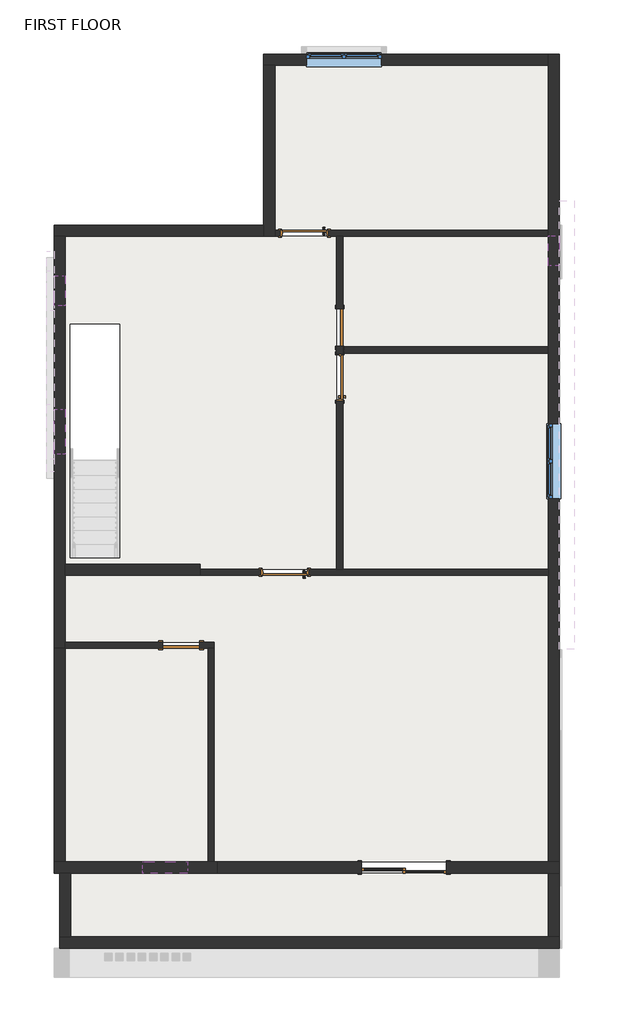
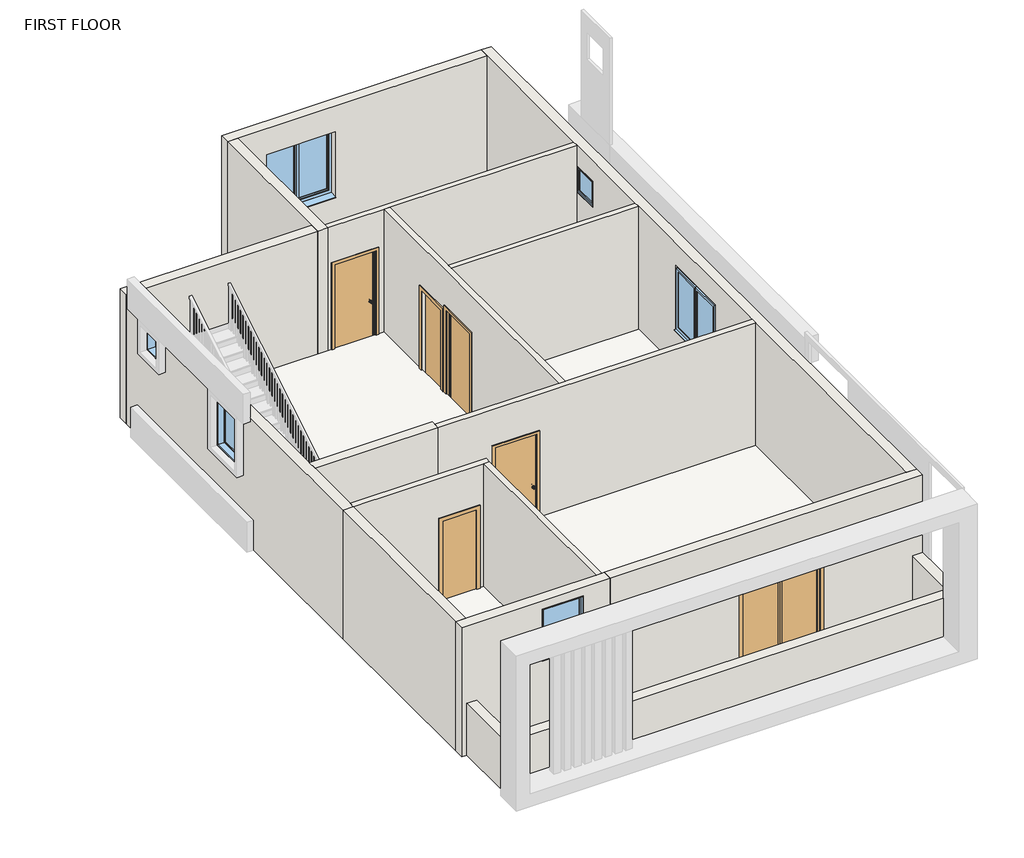
# One storey, part 1 of 2: 18 walls, 6 doors, 6 windows, 1 slab.
"""IFC4 building model written with IfcOpenShell, lengths in millimetres."""

from ifc_helpers import new_model, si_unit, frame, origin, place, context, project, spatial, polyline, outline, extrude, faceted_brep, transform, mapped, element, save
from components import door_45189e27, door_92402058, door_fdc9072e, door_1fe7f57d, window_80340324, fixed_window_3_x_3_dcb239d8, w2_windows_5_x_5_8ac21896

model = new_model("IFC4")

# Units and contexts
model_context = context("Model", 3, world=origin())
ifc_project = project(units=[si_unit("LENGTHUNIT", "METRE", prefix="MILLI")], contexts=[model_context])

# Site, building, storey
site = spatial("IfcSite", under=ifc_project)
building = spatial("IfcBuilding", under=site)
storey = spatial("IfcBuildingStorey", under=building, Name="FIRST FLOOR", Elevation=3352.8)

# Doors
placement = place(None, origin())
door_shape = door_45189e27(model_context)
element("IfcDoor", 1, ObjectType="Door-Double-Sliding : 68\" x 84\"", at=placement, inside=storey, context=model_context, shape_type="MappedRepresentation", body=[
    mapped(door_shape, transform((1027.2719693, -4152.8358748, 3352.8), x_axis=(-1.0, 0.0, 0.0), y_axis=(0.0, -1.0, 0.0), z_axis=(0.0, 0.0, 1.0))),
])
door_2_shape = door_92402058(model_context)
element("IfcDoor", 2, ObjectType="Door-Interior-Single-Flush_Panel-Wood : 36\" x 84\"", at=placement, inside=storey, context=model_context, shape_type="MappedRepresentation", body=[
    mapped(door_2_shape, transform((-1398.4280307, 1724.0891252, 3352.8), x_axis=(-1.0, 0.0, 0.0), y_axis=(0.0, -1.0, 0.0), z_axis=(0.0, 0.0, 1.0))),
])
door_3_shape = door_fdc9072e(model_context)
element("IfcDoor", 3, ObjectType="Door-Interior-Single-Flush_Panel-Wood : 36\" x 84\"", at=placement, inside=storey, context=model_context, shape_type="MappedRepresentation", body=[
    mapped(door_3_shape, transform((-998.3780307, 8626.5391252, 3352.8), x_axis=(-1.0, 0.0, 0.0), y_axis=(0.0, -1.0, 0.0), z_axis=(0.0, 0.0, 1.0))),
])
element("IfcDoor", 4, ObjectType="Door-Interior-Single-Flush_Panel-Wood : 36\" x 84\"", at=placement, inside=storey, context=model_context, shape_type="MappedRepresentation", body=[
    mapped(door_3_shape, transform((-277.6530307, 5689.6641252, 3352.8), x_axis=(0.0, 1.0, 0.0), y_axis=(-1.0, 0.0, 0.0), z_axis=(0.0, 0.0, 1.0))),
])
door_4_shape = door_1fe7f57d(model_context)
element("IfcDoor", 5, ObjectType="Single-Flush : 30\" x 80\"", at=placement, inside=storey, context=model_context, shape_type="MappedRepresentation", body=[
    mapped(door_4_shape, transform((-3509.8822467, 241.3641252, 3352.8), x_axis=(-1.0, 0.0, 0.0), y_axis=(0.0, -1.0, 0.0), z_axis=(0.0, 0.0, 1.0))),
])
element("IfcDoor", 6, ObjectType="Single-Flush : 30\" x 80\"", at=placement, inside=storey, context=model_context, shape_type="MappedRepresentation", body=[
    mapped(door_4_shape, transform((-280.8280307, 6705.6641252, 3352.8), x_axis=(0.0, -1.0, 0.0), y_axis=(1.0, 0.0, 0.0), z_axis=(0.0, 0.0, 1.0))),
])

# Slab
element("IfcSlab", 7, ObjectType="MARBLE 6\"", at=placement, inside=storey, context=model_context, shape_type="SweptSolid", body=[
    extrude(outline(polyline([(-2963.7822467, -4165.5358748), (-5868.7932997, -4165.5358748), (-5868.7932997, 177.8641252), (-2963.7822467, 177.8641252), (-2963.7822467, -4165.5358748)])), frame((0.0, 0.0, 3352.8), z_axis=(0.0, 0.0, 1.0), x_axis=(1.0, 0.0, 0.0)), (0.0, 0.0, 1.0), 152.4),
    extrude(outline(polyline([(-217.3280307, 6184.9641252), (3960.9719693, 6184.9641252), (3960.9719693, 1790.7641252), (-217.3280307, 1790.7641252), (-217.3280307, 6184.9641252)])), frame((0.0, 0.0, 3352.8), z_axis=(0.0, 0.0, 1.0), x_axis=(1.0, 0.0, 0.0)), (0.0, 0.0, 1.0), 152.4),
    extrude(outline(polyline([(-1601.6280307, 12039.6641252), (3960.9719693, 12039.6641252), (3960.9719693, 8686.8641252), (-1601.6280307, 8686.8641252), (-1601.6280307, 12039.6641252)])), frame((0.0, 0.0, 3352.8), z_axis=(0.0, 0.0, 1.0), x_axis=(1.0, 0.0, 0.0)), (0.0, 0.0, 1.0), 152.4),
    extrude(outline(polyline([(-217.3280307, 8559.8641252), (3960.9719693, 8559.8641252), (3960.9719693, 6311.9641252), (-217.3280307, 6311.9641252), (-217.3280307, 8559.8641252)])), frame((0.0, 0.0, 3352.8), z_axis=(0.0, 0.0, 1.0), x_axis=(1.0, 0.0, 0.0)), (0.0, 0.0, 1.0), 152.4),
    extrude(outline(polyline([(3960.9719693, -4394.1358748), (3960.9719693, -5689.5358748), (-5868.7932997, -5689.5358748), (-5868.7932997, -4394.1358748), (3960.9719693, -4394.1358748)])), frame((0.0, 0.0, 3352.8), z_axis=(0.0, 0.0, 1.0), x_axis=(1.0, 0.0, 0.0)), (0.0, 0.0, 1.0), 152.4),
    extrude(outline(polyline([(-344.3280307, 8559.8641252), (-344.3280307, 1790.7641252), (-5868.8280307, 1790.7641252), (-5868.8280307, 8559.8641252), (-344.3280307, 8559.8641252)]), holes=[polyline([(-4756.3875748, 6770.5325341), (-5772.3875748, 6770.5325341), (-5772.3875748, 2020.7325341), (-4756.3875748, 2020.7325341), (-4756.3875748, 6770.5325341)])]), frame((0.0, 0.0, 3352.8), z_axis=(0.0, 0.0, 1.0), x_axis=(1.0, 0.0, 0.0)), (0.0, 0.0, 1.0), 152.4),
    extrude(outline(polyline([(3960.9719693, 1663.7641252), (3960.9719693, -4165.5358748), (-2836.7822467, -4165.5358748), (-2836.7822467, 304.8641252), (-5868.8280307, 304.8641252), (-5868.8280307, 1663.7641252), (3960.9719693, 1663.7641252)])), frame((0.0, 0.0, 3352.8), z_axis=(0.0, 0.0, 1.0), x_axis=(1.0, 0.0, 0.0)), (0.0, 0.0, 1.0), 152.4),
])

# Walls
element("IfcWall", 8, ObjectType="INNER WALL5\"", at=placement, inside=storey, context=model_context, shape_type="Brep", body=[
    faceted_brep([(3960.9719693, 8559.8641252, 6400.8), (-217.3280307, 8559.8641252, 6400.8), (-344.3280307, 8559.8641252, 6400.8), (-1601.6280307, 8559.8641252, 6400.8), (-1601.6280307, 8559.8641252, 3352.8), (-1480.9780307, 8559.8641252, 3352.8), (-1480.9780307, 8559.8641252, 5511.8), (-515.7780307, 8559.8641252, 5511.8), (-515.7780307, 8559.8641252, 3352.8), (-344.3280307, 8559.8641252, 3352.8), (-217.3280307, 8559.8641252, 3352.8), (3960.9719693, 8559.8641252, 3352.8), (-1601.6280307, 8686.8641252, 6400.8), (3960.9719693, 8686.8641252, 6400.8), (3960.9719693, 8686.8641252, 3352.8), (-515.7780307, 8686.8641252, 3352.8), (-515.7780307, 8686.8641252, 5511.8), (-1480.9780307, 8686.8641252, 5511.8), (-1480.9780307, 8686.8641252, 3352.8), (-1601.6280307, 8686.8641252, 3352.8)], [[[0, 1, 2, 3, 4, 5, 6, 7, 8, 9, 10, 11]], [[12, 13, 14, 15, 16, 17, 18, 19]], [[14, 11, 10, 9, 8, 15]], [[4, 19, 18, 5]], [[3, 2, 1, 0, 13, 12]], [[0, 11, 14, 13]], [[4, 3, 12, 19]], [[17, 6, 5, 18]], [[6, 17, 16, 7]], [[7, 16, 15, 8]]]),
])
element("IfcWall", 9, ObjectType="INNER WALL5\"", at=placement, inside=storey, context=model_context, shape_type="Brep", body=[
    faceted_brep([(-5868.7932997, 177.8641252, 3352.8), (-3890.8822467, 177.8641252, 3352.8), (-3890.8822467, 177.8641252, 5384.8), (-3128.8822467, 177.8641252, 5384.8), (-3128.8822467, 177.8641252, 3352.8), (-2963.7822467, 177.8641252, 3352.8), (-2836.7822467, 177.8641252, 3352.8), (-2836.7822467, 177.8641252, 6400.8), (-2963.7822467, 177.8641252, 6400.8), (-5868.7932997, 177.8641252, 6400.8), (-3890.8822467, 304.8641252, 5384.8), (-3890.8822467, 304.8641252, 3352.8), (-5868.7932997, 304.8641252, 3352.8), (-5868.7932997, 304.8641252, 6400.8), (-2836.7822467, 304.8641252, 6400.8), (-2836.7822467, 304.8641252, 3352.8), (-3128.8822467, 304.8641252, 3352.8), (-3128.8822467, 304.8641252, 5384.8)], [[[0, 1, 2, 3, 4, 5, 6, 7, 8, 9]], [[10, 11, 12, 13, 14, 15, 16, 17]], [[16, 15, 6, 5, 4]], [[12, 11, 1, 0]], [[9, 8, 7, 14, 13]], [[7, 6, 15, 14]], [[2, 1, 11, 10]], [[3, 2, 10, 17]], [[4, 3, 17, 16]], [[0, 9, 13, 12]]]),
])
element("IfcWall", 10, ObjectType="INNER WALL5\"", at=placement, inside=storey, context=model_context, shape_type="SweptSolid", body=[
    extrude(outline(polyline([(-2963.7822467, -4165.5358748), (-2963.7822467, 177.8641252), (-2836.7822467, 177.8641252), (-2836.7822467, -4165.5358748), (-2963.7822467, -4165.5358748)])), frame((0.0, 0.0, 3352.8), z_axis=(0.0, 0.0, 1.0), x_axis=(1.0, 0.0, 0.0)), (0.0, 0.0, 1.0), 3048.0),
])
element("IfcWall", 11, ObjectType="INNER WALL5\"", at=placement, inside=storey, context=model_context, shape_type="Brep", body=[
    faceted_brep([(3960.9719693, 1663.7641252, 6400.8), (-3125.6280307, 1663.7641252, 6400.8), (-3125.6280307, 1663.7641252, 3352.8), (-1881.0280307, 1663.7641252, 3352.8), (-1881.0280307, 1663.7641252, 5511.8), (-915.8280307, 1663.7641252, 5511.8), (-915.8280307, 1663.7641252, 3352.8), (3960.9719693, 1663.7641252, 3352.8), (-3125.6280307, 1790.7641252, 6400.8), (-344.3280307, 1790.7641252, 6400.8), (-217.3280307, 1790.7641252, 6400.8), (3960.9719693, 1790.7641252, 6400.8), (3960.9719693, 1790.7641252, 3352.8), (-217.3280307, 1790.7641252, 3352.8), (-344.3280307, 1790.7641252, 3352.8), (-915.8280307, 1790.7641252, 3352.8), (-915.8280307, 1790.7641252, 5511.8), (-1881.0280307, 1790.7641252, 5511.8), (-1881.0280307, 1790.7641252, 3352.8), (-3125.6280307, 1790.7641252, 3352.8)], [[[0, 1, 2, 3, 4, 5, 6, 7]], [[8, 9, 10, 11, 12, 13, 14, 15, 16, 17, 18, 19]], [[2, 19, 18, 3]], [[12, 7, 6, 15, 14, 13]], [[1, 0, 11, 10, 9, 8]], [[2, 1, 8, 19]], [[0, 7, 12, 11]], [[17, 4, 3, 18]], [[4, 17, 16, 5]], [[5, 16, 15, 6]]]),
])
element("IfcWall", 12, ObjectType="INNER WALL5\"", at=placement, inside=storey, context=model_context, shape_type="Brep", body=[
    faceted_brep([(-344.3280307, 1790.7641252, 6400.8), (-344.3280307, 8559.8641252, 6400.8), (-344.3280307, 8559.8641252, 3352.8), (-344.3280307, 7086.6641252, 3352.8), (-344.3280307, 7086.6641252, 5384.8), (-344.3280307, 6324.6641252, 5384.8), (-344.3280307, 6324.6641252, 3352.8), (-344.3280307, 6172.2641252, 3352.8), (-344.3280307, 6172.2641252, 5511.8), (-344.3280307, 5207.0641252, 5511.8), (-344.3280307, 5207.0641252, 3352.8), (-344.3280307, 1790.7641252, 3352.8), (-217.3280307, 8559.8641252, 6400.8), (-217.3280307, 6311.9641252, 6400.8), (-217.3280307, 6184.9641252, 6400.8), (-217.3280307, 1790.7641252, 6400.8), (-217.3280307, 1790.7641252, 3352.8), (-217.3280307, 5207.0641252, 3352.8), (-217.3280307, 5207.0641252, 5511.8), (-217.3280307, 6172.2641252, 5511.8), (-217.3280307, 6172.2641252, 3352.8), (-217.3280307, 6184.9641252, 3352.8), (-217.3280307, 6311.9641252, 3352.8), (-217.3280307, 6324.6641252, 3352.8), (-217.3280307, 6324.6641252, 5384.8), (-217.3280307, 7086.6641252, 5384.8), (-217.3280307, 7086.6641252, 3352.8), (-217.3280307, 8559.8641252, 3352.8)], [[[0, 1, 2, 3, 4, 5, 6, 7, 8, 9, 10, 11]], [[12, 13, 14, 15, 16, 17, 18, 19, 20, 21, 22, 23, 24, 25, 26, 27]], [[2, 27, 26, 3]], [[16, 11, 10, 17]], [[6, 23, 22, 21, 20, 7]], [[1, 0, 15, 14, 13, 12]], [[2, 1, 12, 27]], [[0, 11, 16, 15]], [[24, 23, 6, 5]], [[25, 24, 5, 4]], [[26, 25, 4, 3]], [[19, 8, 7, 20]], [[8, 19, 18, 9]], [[9, 18, 17, 10]]]),
])
element("IfcWall", 13, ObjectType="INNER WALL5\"", at=placement, inside=storey, context=model_context, shape_type="SweptSolid", body=[
    extrude(outline(polyline([(3960.9719693, 6184.9641252), (-217.3280307, 6184.9641252), (-217.3280307, 6311.9641252), (3960.9719693, 6311.9641252), (3960.9719693, 6184.9641252)])), frame((0.0, 0.0, 3352.8), z_axis=(0.0, 0.0, 1.0), x_axis=(1.0, 0.0, 0.0)), (0.0, 0.0, 1.0), 3048.0),
])
element("IfcWall", 14, ObjectType="OUTER WALL 9\"", at=placement, inside=storey, context=model_context, shape_type="Brep", body=[
    faceted_brep([(4189.5719693, -4165.5358748, 6400.8), (4189.5719693, -4165.5358748, 3352.8), (4189.5719693, 12268.2641252, 3352.8), (4189.5719693, 12268.2641252, 6400.8), (4189.5719693, 4749.8641252, 4352.8), (4189.5719693, 3225.8641252, 4352.8), (4189.5719693, 3225.8641252, 5876.8), (4189.5719693, 4749.8641252, 5876.8), (4189.5719693, 8572.5641252, 5908.2819261), (4189.5719693, 8572.5641252, 5298.6819261), (4189.5719693, 7962.9641252, 5298.6819261), (4189.5719693, 7962.9641252, 5908.2819261), (3960.9719693, -4165.5358748, 3352.8), (3960.9719693, -4165.5358748, 6400.8), (3960.9719693, 1663.7641252, 6400.8), (3960.9719693, 1790.7641252, 6400.8), (3960.9719693, 6184.9641252, 6400.8), (3960.9719693, 6311.9641252, 6400.8), (3960.9719693, 8559.8641252, 6400.8), (3960.9719693, 8686.8641252, 6400.8), (3960.9719693, 12039.6641252, 6400.8), (3960.9719693, 12268.2641252, 6400.8), (3960.9719693, 12268.2641252, 3352.8), (3960.9719693, 12039.6641252, 3352.8), (3960.9719693, 8686.8641252, 3352.8), (3960.9719693, 8559.8641252, 3352.8), (3960.9719693, 6311.9641252, 3352.8), (3960.9719693, 6184.9641252, 3352.8), (3960.9719693, 1790.7641252, 3352.8), (3960.9719693, 1663.7641252, 3352.8), (3960.9719693, 4749.8641252, 4352.8), (3960.9719693, 4749.8641252, 5876.8), (3960.9719693, 3225.8641252, 5876.8), (3960.9719693, 3225.8641252, 4352.8), (3960.9719693, 8572.5641252, 5908.2819261), (3960.9719693, 7962.9641252, 5908.2819261), (3960.9719693, 7962.9641252, 5298.6819261), (3960.9719693, 8572.5641252, 5298.6819261)], [[[0, 1, 2, 3], [4, 5, 6, 7], [8, 9, 10, 11]], [[12, 13, 14, 15, 16, 17, 18, 19, 20, 21, 22, 23, 24, 25, 26, 27, 28, 29], [30, 31, 32, 33], [34, 35, 36, 37]], [[2, 1, 12, 29, 28, 27, 26, 25, 24, 23, 22]], [[0, 3, 21, 20, 19, 18, 17, 16, 15, 14, 13]], [[3, 2, 22, 21]], [[0, 13, 12, 1]], [[31, 30, 4, 7]], [[32, 31, 7, 6]], [[33, 32, 6, 5]], [[30, 33, 5, 4]], [[9, 8, 34, 37]], [[10, 9, 37, 36]], [[11, 10, 36, 35]], [[8, 11, 35, 34]]]),
])
element("IfcWall", 15, ObjectType="OUTER WALL 9\"", at=placement, inside=storey, context=model_context, shape_type="Brep", body=[
    faceted_brep([(3960.9719693, 12268.2641252, 3352.8), (-1830.2280307, 12268.2641252, 3352.8), (-1830.2280307, 12268.2641252, 6400.8), (3960.9719693, 12268.2641252, 6400.8), (570.0719693, 12268.2641252, 4267.2), (570.0719693, 12268.2641252, 5791.2), (-953.9280307, 12268.2641252, 5791.2), (-953.9280307, 12268.2641252, 4267.2), (3960.9719693, 12039.6641252, 3352.8), (3960.9719693, 12039.6641252, 6400.8), (-1601.6280307, 12039.6641252, 6400.8), (-1830.2280307, 12039.6641252, 6400.8), (-1830.2280307, 12039.6641252, 3352.8), (-1601.6280307, 12039.6641252, 3352.8), (570.0719693, 12039.6641252, 4267.2), (-953.9280307, 12039.6641252, 4267.2), (-953.9280307, 12039.6641252, 5791.2), (570.0719693, 12039.6641252, 5791.2)], [[[0, 1, 2, 3], [4, 5, 6, 7]], [[8, 9, 10, 11, 12, 13], [14, 15, 16, 17]], [[1, 0, 8, 13, 12]], [[3, 2, 11, 10, 9]], [[0, 3, 9, 8]], [[2, 1, 12, 11]], [[5, 4, 14, 17]], [[6, 5, 17, 16]], [[7, 6, 16, 15]], [[4, 7, 15, 14]]]),
])
element("IfcWall", 16, ObjectType="OUTER WALL 9\"", at=placement, inside=storey, context=model_context, shape_type="Brep", body=[
    faceted_brep([(-1830.2280307, 12039.6641252, 3352.8), (-1830.2280307, 8788.4641252, 3352.8), (-1830.2280307, 8559.8641252, 3352.8), (-1830.2280307, 8559.8641252, 6400.8), (-1830.2280307, 8788.4641252, 6400.8), (-1830.2280307, 12039.6641252, 6400.8), (-1601.6280307, 12039.6641252, 3352.8), (-1601.6280307, 12039.6641252, 6400.8), (-1601.6280307, 8686.8641252, 6400.8), (-1601.6280307, 8559.8641252, 6400.8), (-1601.6280307, 8559.8641252, 3352.8), (-1601.6280307, 8686.8641252, 3352.8)], [[[0, 1, 2, 3, 4, 5]], [[6, 7, 8, 9, 10, 11]], [[2, 1, 0, 6, 11, 10]], [[5, 4, 3, 9, 8, 7]], [[0, 5, 7, 6]], [[3, 2, 10, 9]]]),
])
element("IfcWall", 17, ObjectType="OUTER WALL 9\"", at=placement, inside=storey, context=model_context, shape_type="Brep", body=[
    faceted_brep([(-1830.2280307, 8788.4641252, 3352.8), (-6097.3932997, 8788.4641252, 3352.8), (-6097.3932997, 8788.4641252, 6400.8), (-1830.2280307, 8788.4641252, 6400.8), (-1830.2280307, 8559.8641252, 3352.8), (-1830.2280307, 8559.8641252, 6400.8), (-5868.7932997, 8559.8641252, 6400.8), (-6097.3932997, 8559.8641252, 6400.8), (-6097.3932997, 8559.8641252, 3352.8), (-5868.7932997, 8559.8641252, 3352.8)], [[[0, 1, 2, 3]], [[4, 5, 6, 7, 8, 9]], [[1, 0, 4, 9, 8]], [[3, 2, 7, 6, 5]], [[0, 3, 5, 4]], [[2, 1, 8, 7]]]),
])
element("IfcWall", 18, ObjectType="OUTER WALL 9\"", at=placement, inside=storey, context=model_context, shape_type="Brep", body=[
    faceted_brep([(-6097.3932997, 8559.8641252, 3352.8), (-6097.3932997, 177.8641252, 3352.8), (-6097.3932997, 177.8641252, 6400.8), (-6097.3932997, 8559.8641252, 6400.8), (-6097.3932997, 7150.1641252, 6189.9849297), (-6097.3932997, 7150.1641252, 5580.3849297), (-6097.3932997, 7759.7641252, 5580.3849297), (-6097.3932997, 7759.7641252, 6189.9849297), (-6097.3932997, 4127.5641252, 6204.2433359), (-6097.3932997, 4127.5641252, 4985.0433359), (-6097.3932997, 5041.9641252, 4985.0433359), (-6097.3932997, 5041.9641252, 6204.2433359), (-5868.7932997, 8559.8641252, 3352.8), (-5868.7932997, 8559.8641252, 6400.8), (-5868.7932997, 1892.3641252, 6400.8), (-5868.7932997, 1663.7641252, 6400.8), (-5868.7932997, 304.8641252, 6400.8), (-5868.7932997, 177.8641252, 6400.8), (-5868.7932997, 177.8641252, 3352.8), (-5868.7932997, 304.8641252, 3352.8), (-5868.7932997, 1663.7641252, 3352.8), (-5868.7932997, 1892.3641252, 3352.8), (-5868.7932997, 7150.1641252, 6189.9849297), (-5868.7932997, 7759.7641252, 6189.9849297), (-5868.7932997, 7759.7641252, 5580.3849297), (-5868.7932997, 7150.1641252, 5580.3849297), (-5868.7932997, 4127.5641252, 6204.2433359), (-5868.7932997, 5041.9641252, 6204.2433359), (-5868.7932997, 5041.9641252, 4985.0433359), (-5868.7932997, 4127.5641252, 4985.0433359)], [[[0, 1, 2, 3], [4, 5, 6, 7], [8, 9, 10, 11]], [[12, 13, 14, 15, 16, 17, 18, 19, 20, 21], [22, 23, 24, 25], [26, 27, 28, 29]], [[1, 0, 12, 21, 20, 19, 18]], [[3, 2, 17, 16, 15, 14, 13]], [[0, 3, 13, 12]], [[2, 1, 18, 17]], [[5, 4, 22, 25]], [[6, 5, 25, 24]], [[7, 6, 24, 23]], [[4, 7, 23, 22]], [[9, 8, 26, 29]], [[10, 9, 29, 28]], [[11, 10, 28, 27]], [[8, 11, 27, 26]]]),
])
element("IfcWall", 19, ObjectType="OUTER WALL 9\"", at=placement, inside=storey, context=model_context, shape_type="Brep", body=[
    faceted_brep([(-2782.7280307, -4394.1358748, 3352.8), (163.6719693, -4394.1358748, 3352.8), (163.6719693, -4394.1358748, 5486.4), (1890.8719693, -4394.1358748, 5486.4), (1890.8719693, -4394.1358748, 3352.8), (3960.9719693, -4394.1358748, 3352.8), (4189.5719693, -4394.1358748, 3352.8), (4189.5719693, -4394.1358748, 4572.0), (4189.5719693, -4394.1358748, 6400.8), (-2782.7280307, -4394.1358748, 6400.8), (163.6719693, -4165.5358748, 5486.4), (163.6719693, -4165.5358748, 3352.8), (-2782.7280307, -4165.5358748, 3352.8), (-2782.7280307, -4165.5358748, 6400.8), (3960.9719693, -4165.5358748, 6400.8), (4189.5719693, -4165.5358748, 6400.8), (4189.5719693, -4165.5358748, 3352.8), (3960.9719693, -4165.5358748, 3352.8), (1890.8719693, -4165.5358748, 3352.8), (1890.8719693, -4165.5358748, 5486.4)], [[[0, 1, 2, 3, 4, 5, 6, 7, 8, 9]], [[10, 11, 12, 13, 14, 15, 16, 17, 18, 19]], [[12, 11, 1, 0]], [[18, 17, 16, 6, 5, 4]], [[9, 8, 15, 14, 13]], [[0, 9, 13, 12]], [[6, 16, 15, 8, 7]], [[4, 3, 19, 18]], [[2, 1, 11, 10]], [[3, 2, 10, 19]]]),
])
element("IfcWall", 20, ObjectType="OUTER WALL 9\"", at=placement, inside=storey, context=model_context, shape_type="Brep", body=[
    faceted_brep([(-2782.7280307, -4165.5358748, 3352.8), (-2836.7822467, -4165.5358748, 3352.8), (-2963.7822467, -4165.5358748, 3352.8), (-5868.7932997, -4165.5358748, 3352.8), (-6097.3932997, -4165.5358748, 3352.8), (-6097.3932997, -4165.5358748, 6400.8), (-5868.7932997, -4165.5358748, 6400.8), (-2963.7822467, -4165.5358748, 6400.8), (-2836.7822467, -4165.5358748, 6400.8), (-2782.7280307, -4165.5358748, 6400.8), (-4294.0280307, -4165.5358748, 6197.6), (-4294.0280307, -4165.5358748, 4978.4), (-3379.6280307, -4165.5358748, 4978.4), (-3379.6280307, -4165.5358748, 6197.6), (-2782.7280307, -4394.1358748, 3352.8), (-2782.7280307, -4394.1358748, 6400.8), (-6097.3932997, -4394.1358748, 6400.8), (-6097.3932997, -4394.1358748, 3352.8), (-5983.1280307, -4394.1358748, 3352.8), (-5754.5280307, -4394.1358748, 3352.8), (-4294.0280307, -4394.1358748, 6197.6), (-3379.6280307, -4394.1358748, 6197.6), (-3379.6280307, -4394.1358748, 4978.4), (-4294.0280307, -4394.1358748, 4978.4)], [[[0, 1, 2, 3, 4, 5, 6, 7, 8, 9], [10, 11, 12, 13]], [[14, 15, 16, 17, 18, 19], [20, 21, 22, 23]], [[4, 3, 2, 1, 0, 14, 19, 18, 17]], [[9, 8, 7, 6, 5, 16, 15]], [[0, 9, 15, 14]], [[11, 10, 20, 23]], [[12, 11, 23, 22]], [[13, 12, 22, 21]], [[10, 13, 21, 20]], [[4, 17, 16, 5]]]),
])
element("IfcWall", 21, ObjectType="OUTER WALL 9\"", at=placement, inside=storey, context=model_context, shape_type="Brep", body=[
    faceted_brep([(-5983.1280307, -5918.1358748, 3352.8), (4189.5719693, -5918.1358748, 3352.8), (4189.5719693, -5918.1358748, 4572.0), (-5983.1280307, -5918.1358748, 4572.0), (-5983.1280307, -5689.5358748, 3352.8), (-5983.1280307, -5689.5358748, 4572.0), (-5754.5280307, -5689.5358748, 4572.0), (3960.9719693, -5689.5358748, 4572.0), (4189.5719693, -5689.5358748, 4572.0), (4189.5719693, -5689.5358748, 3352.8), (3960.9719693, -5689.5358748, 3352.8), (-5754.5280307, -5689.5358748, 3352.8)], [[[0, 1, 2, 3]], [[4, 5, 6, 7, 8, 9, 10, 11]], [[1, 0, 4, 11, 10, 9]], [[3, 2, 8, 7, 6, 5]], [[2, 1, 9, 8]], [[0, 3, 5, 4]]]),
])
element("IfcWall", 22, ObjectType="OUTER WALL 9\"", at=placement, inside=storey, context=model_context, shape_type="SweptSolid", body=[
    extrude(outline(polyline([(3960.9719693, -5689.5358748), (3960.9719693, -4394.1358748), (4189.5719693, -4394.1358748), (4189.5719693, -5689.5358748), (3960.9719693, -5689.5358748)])), frame((0.0, 0.0, 3352.8), z_axis=(0.0, 0.0, 1.0), x_axis=(1.0, 0.0, 0.0)), (0.0, 0.0, 1.0), 1219.2),
])
element("IfcWall", 23, ObjectType="OUTER WALL 9\"", at=placement, inside=storey, context=model_context, shape_type="Brep", body=[
    faceted_brep([(-5868.7932997, 1663.7641252, 3352.8), (-3125.6280307, 1663.7641252, 3352.8), (-3125.6280307, 1663.7641252, 6400.8), (-5868.7932997, 1663.7641252, 6400.8), (-5868.7932997, 1892.3641252, 3352.8), (-5868.7932997, 1892.3641252, 6400.8), (-3125.6280307, 1892.3641252, 6400.8), (-3125.6280307, 1892.3641252, 3352.8), (-3125.6280307, 1790.7641252, 3352.8), (-3125.6280307, 1790.7641252, 6400.8)], [[[0, 1, 2, 3]], [[4, 5, 6, 7]], [[1, 0, 4, 7, 8]], [[2, 1, 8, 7, 6, 9]], [[3, 2, 9, 6, 5]], [[0, 3, 5, 4]]]),
])
element("IfcWall", 24, ObjectType="OUTER WALL 9\"", at=placement, inside=storey, context=model_context, shape_type="SweptSolid", body=[
    extrude(outline(polyline([(-5983.1280307, -5689.5358748), (-5983.1280307, -4394.1358748), (-5754.5280307, -4394.1358748), (-5754.5280307, -5689.5358748), (-5983.1280307, -5689.5358748)])), frame((0.0, 0.0, 3352.8), z_axis=(0.0, 0.0, 1.0), x_axis=(1.0, 0.0, 0.0)), (0.0, 0.0, 1.0), 1219.2),
])
element("IfcWall", 25, ObjectType="OUTER WALL 9\"", at=placement, inside=storey, context=model_context, shape_type="SweptSolid", body=[
    extrude(outline(polyline([(-6097.3932997, -4165.5358748), (-6097.3932997, 177.8641252), (-5868.7932997, 177.8641252), (-5868.7932997, -4165.5358748), (-6097.3932997, -4165.5358748)])), frame((0.0, 0.0, 3352.8), z_axis=(0.0, 0.0, 1.0), x_axis=(1.0, 0.0, 0.0)), (0.0, 0.0, 1.0), 3048.0),
])

# Windows
window_shape = window_80340324(model_context)
element("IfcWindow", 26, ObjectType="Fixed : 24\" x 24\"", at=placement, inside=storey, context=model_context, shape_type="MappedRepresentation", body=[
    mapped(window_shape, transform((4075.2719693, 8305.8641252, 4384.2819261), x_axis=(0.0, 1.0, 0.0), y_axis=(-1.0, 0.0, 0.0), z_axis=(0.0, 0.0, 1.0))),
])
element("IfcWindow", 27, ObjectType="Fixed : 24\" x 24\"", at=placement, inside=storey, context=model_context, shape_type="MappedRepresentation", body=[
    mapped(window_shape, transform((-5983.0932997, 7416.8641252, 4665.9849297), x_axis=(0.0, -1.0, 0.0), y_axis=(1.0, 0.0, 0.0), z_axis=(0.0, 0.0, 1.0))),
])
fixed_window_3_x_3_shape = fixed_window_3_x_3_dcb239d8(model_context)
element("IfcWindow", 28, ObjectType="Fixed : window 3' x 3'", at=placement, inside=storey, context=model_context, shape_type="MappedRepresentation", body=[
    mapped(fixed_window_3_x_3_shape, transform((-3874.9280307, -4279.8358748, 4064.0), x_axis=(-1.0, 0.0, 0.0), y_axis=(0.0, -1.0, 0.0), z_axis=(0.0, 0.0, 1.0))),
])
element("IfcWindow", 29, ObjectType="Fixed : window 3' x 3'", at=placement, inside=storey, context=model_context, shape_type="MappedRepresentation", body=[
    mapped(fixed_window_3_x_3_shape, transform((-5983.0932997, 4546.6641252, 4070.6433359), x_axis=(0.0, -1.0, 0.0), y_axis=(1.0, 0.0, 0.0), z_axis=(0.0, 0.0, 1.0))),
])
w2_windows_5_x_5_shape = w2_windows_5_x_5_8ac21896(model_context)
element("IfcWindow", 30, ObjectType="w2 : WINDOWS 5' X 5'", at=placement, inside=storey, context=model_context, shape_type="MappedRepresentation", body=[
    mapped(w2_windows_5_x_5_shape, transform((4075.2719693, 3987.8641252, 3352.8), x_axis=(0.0, -1.0, 0.0), y_axis=(1.0, 0.0, 0.0), z_axis=(0.0, 0.0, 1.0))),
])
element("IfcWindow", 31, ObjectType="w2 : WINDOWS 5' X 5'", at=placement, inside=storey, context=model_context, shape_type="MappedRepresentation", body=[
    mapped(w2_windows_5_x_5_shape, transform((-191.9280307, 12153.9641252, 3267.2), x_axis=(-1.0, 0.0, 0.0), y_axis=(0.0, -1.0, 0.0), z_axis=(0.0, 0.0, 1.0))),
])

save(model, "model.ifc")

# Revit data of these elements
# Type "Door-Double-Sliding : 68\" x 84\""
#   Type Mark = "9"
#   Construction Type Id = "opn-d45"
#   Assembly Code = "C1020"
#   Analytic Construction = "Wood frame, double glass door "
#   Thickness = 0' - 2"
#   Thermal Resistance (R) = 1.8150 (h·ft²·°F)/BTU
#   Heat Transfer Coefficient (U) = 0.5510 BTU/(h·ft²·°F)
#   Height = 7' - 0"
#   Rail Width = 0' - 2"
#   Stiles = 0' - 2"
#   Trim Projection Ext = 0' - 1"
#   Trim Projection Int = 0' - 1"
#   Trim Width = 0' - 3"
#   Width = 5' - 8"
#   Define Thermal Properties by = 1
#   Glazing = Glass
#   Panel Material = Wood - Birch - Solid Stained Light Low Gloss
#   Trim Material = Paint - Sienna
#   Visual Light Transmittance = 0
#   Solar Heat Gain Coefficient = 0
#   Function = (empty or 0)
#   Wall Closure = (empty or 0)
# Type "Door-Interior-Single-Flush_Panel-Wood : 36\" x 84\""
#   Type Mark = "8"
#   Assembly Code = "C1020300"
#   Analytic Construction = "Wooden"
#   Thickness = 0' - 1 3/8"
#   Thermal Resistance (R) = 2.5876 (h·ft²·°F)/BTU
#   Swing Angle [instance default] = 90.00°
#   Rough Width = 3' - 2"
#   Rough Height = 7' - 1"
#   Height = 7' - 0"
#   Width = 3' - 0"
#   Heat Transfer Coefficient (U) = 0.3865 BTU/(h·ft²·°F)
#   Trim Material = Cherry
#   Panel Material = Cherry
#   Frame Material = Cherry
#   Door Handle Material = Aluminum
#   Visual Light Transmittance = 0
#   Solar Heat Gain Coefficient = 0
#   Wall Closure = (empty or 0)
#   Function = (empty or 0)
# Type "Single-Flush : 30\" x 80\""
#   Type Mark = "5"
#   Construction Type Id = "MDOOR"
#   Assembly Code = "C1020"
#   Analytic Construction = "Metal"
#   Thickness = 0' - 2"
#   Heat Transfer Coefficient (U) = 0.651978 BTU/(h·ft²·°F)
#   Height = 6' - 8"
#   Trim Projection Ext = 0' - 1"
#   Trim Projection Int = 0' - 1"
#   Trim Width = 0' - 3"
#   Width = 2' - 6"
#   Define Thermal Properties by = 1
#   Define Thermal Properties by = 1
#   Door Material = Door - Panel
#   Frame Material = Door - Frame
#   Visual Light Transmittance = 0
#   Solar Heat Gain Coefficient = 0
#   Function = (empty or 0)
#   Wall Closure = (empty or 0)
# Type "MARBLE 6\""
#   Assembly Code = "B1010"
#   Function = 0
#   Layers, outside or top first: 0' - 6" "MARBLE MATERIAL" (function 1)
# Type "INNER WALL5\""
#   Assembly Code = "B2010"
#   Layers, outside or top first: 0' - 5" "OUTER WALL 9\"" (function 1)
# Type "OUTER WALL 9\""
#   Assembly Code = "B2010"
#   Layers, outside or top first: 0' - 9" "OUTER WALL 9\"" (function 1)
# Type "Fixed : 24\" x 24\""
#   Type Mark = "3"
#   Construction Type Id = "GSP4R"
#   Assembly Code = "B2020100"
#   Analytic Construction = "1/8 in Pilkington single glazing"
#   Visual Light Transmittance = 0.9
#   Solar Heat Gain Coefficient = 0.78
#   Heat Transfer Coefficient (U) = 0.6496 BTU/(h·ft²·°F)
#   Height = 2' - 0"
#   Default Sill Height = 3' - 0"
#   Width = 2' - 0"
#   Window Inset = 0' - 0 3/4"
#   Define Thermal Properties by = 1
#   Define Thermal Properties by = 1
#   Glass Pane Material = Glass
#   Sash Material = Sash
#   Wall Closure = (empty or 0)
# Type "Fixed : window 3' x 3'"
#   Type Mark = "18"
#   Construction Type Id = "GSP4R"
#   Assembly Code = "B2020100"
#   Analytic Construction = "1/8 in Pilkington single glazing"
#   Visual Light Transmittance = 0.9
#   Solar Heat Gain Coefficient = 0.78
#   Heat Transfer Coefficient (U) = 0.6496 BTU/(h·ft²·°F)
#   Height = 4' - 0"
#   Default Sill Height = 3' - 0"
#   Width = 3' - 0"
#   Window Inset = 0' - 2"
#   Define Thermal Properties by = 1
#   Glass Pane Material = Glass
#   Sash Material = Sash
#   Wall Closure = (empty or 0)
# Type "w2 : WINDOWS 5' X 5'"
#   Type Mark = "26"
#   Operation = "DoublePanelVertical"
#   Keynote = "16.05.01"
#   Analytic Construction = "<None>"
#   Rough Width = 5' - 0"
#   Rough Height = 5' - 0"
#   Rahmentiefe = 0' - 2.3622"
#   Rahmenhöhe unten = 0' - 3.14961"
#   Rahmehöhe oben = 0' - 3.14961"
#   Rahmenbreite = 0' - 2.3622"
#   Heat Transfer Coefficient (U) = 2.81836 BTU/(h·ft²·°F)
#   Height = 5' - 0"
#   Flügeltiefe = 0' - 2.3622"
#   Flügelbreite = 0' - 2.3622"
#   Einbautiefe (von außen) [instance default] = 0' - 5.51181"
#   Width = 5' - 0"
#   Kippflügel [instance default] = yes
#   Drehflügel im Grundriß darstellen [instance default] = no
#   Drehflügel [instance default] = yes
#   Define Thermal Properties by = 1
#   Rahmen [instance default] = none
#   Glas [instance default] = blue glass
#   Flügel [instance default] = WINDOW COLOUR WHITE
#   Fensterbank aussen [instance default] = WINDOW COLOUR WHITE
#   Fensterbank innen [instance default] = WINDOW COLOUR WHITE
#   Visual Light Transmittance = 0
#   Thermal Resistance (R) = 0
#   Solar Heat Gain Coefficient = 0
#   Wall Closure = (empty or 0)
# Element 1 (IfcDoor, "Door-Double-Sliding : 68\" x 84\"")
#   Phase Created = New Construction
#   Materials on its faces: "Paint - Sienna", "Wood - Birch - Solid Stained Light Low Gloss", "Glass"
# Elements 2, 3, 4 (IfcDoor, "Door-Interior-Single-Flush_Panel-Wood : 36\" x 84\"")
#   Swing Angle = 90.00°
#   Phase Created = New Construction
#   Materials on its faces: "Cherry", "Aluminum"
# Elements 5, 6 (IfcDoor, "Single-Flush : 30\" x 80\"")
#   Phase Created = New Construction
#   Materials on its faces: "Door - Frame", "Door - Panel"
# Element 7 (IfcSlab, "MARBLE 6\"")
#   Height Offset From Level = 0' - 6"
#   Phase Created = New Construction
#   Materials on its faces: "MARBLE MATERIAL"
# Elements 8, 9, 10, 11, 12, 13 (IfcWall, "INNER WALL5\"")
#   Top Offset = 0' - 0"
#   Base Offset = 0' - 0"
#   wall height = 10' - 0"
#   Phase Created = New Construction
#   Base Constraint = FIRST FLOOR
#   Top Constraint = SECOND FLR
#   Materials on its faces: "OUTER WALL 9\""
# Elements 14, 15, 16, 17, 18, 19, 20, 23 (IfcWall, "OUTER WALL 9\"")
#   Top Offset = 0' - 0"
#   Base Offset = 0' - 0"
#   wall height = 10' - 0"
#   Phase Created = New Construction
#   Base Constraint = FIRST FLOOR
#   Top Constraint = SECOND FLR
#   Materials on its faces: "OUTER WALL 9\""
# Elements 21, 22 (IfcWall, "OUTER WALL 9\"")
#   Top Offset = -6' - 0"
#   Base Offset = 0' - 0"
#   wall height = 4' - 0"
#   Phase Created = New Construction
#   Base Constraint = FIRST FLOOR
#   Top Constraint = SECOND FLR
#   Materials on its faces: "OUTER WALL 9\""
# Element 24 (IfcWall, "OUTER WALL 9\"")
#   Top Offset = 0' - 0"
#   Base Offset = 0' - 0"
#   Unconnected Height = 4' - 0"
#   wall height = 4' - 0"
#   Phase Created = New Construction
#   Base Constraint = FIRST FLOOR
#   Materials on its faces: "OUTER WALL 9\""
# Element 25 (IfcWall, "OUTER WALL 9\"")
#   Top Offset = 0' - 0"
#   Base Offset = 0' - 0"
#   Unconnected Height = 10' - 0"
#   wall height = 10' - 0"
#   Phase Created = New Construction
#   Base Constraint = FIRST FLOOR
#   Materials on its faces: "OUTER WALL 9\""
# Element 26 (IfcWindow, "Fixed : 24\" x 24\"")
#   Mark = "7"
#   Phase Created = New Construction
#   Materials on its faces: "Sash", "Glass"
# Element 27 (IfcWindow, "Fixed : 24\" x 24\"")
#   Mark = "12"
#   Phase Created = New Construction
#   Materials on its faces: "Sash", "Glass"
# Element 28 (IfcWindow, "Fixed : window 3' x 3'")
#   Mark = "1"
#   Phase Created = New Construction
#   Materials on its faces: "Sash", "Glass"
# Element 29 (IfcWindow, "Fixed : window 3' x 3'")
#   Mark = "16"
#   Phase Created = New Construction
#   Materials on its faces: "Sash", "Glass"
# Element 30 (IfcWindow, "w2 : WINDOWS 5' X 5'")
#   Mark = "4"
#   Einbautiefe (von außen) = 0' - 5.51181"
#   Kippflügel = yes
#   Drehflügel im Grundriß darstellen = no
#   Drehflügel = yes
#   Rahmen = none
#   Glas = blue glass
#   Flügel = WINDOW COLOUR WHITE
#   Fensterbank innen = WINDOW COLOUR WHITE
#   Fensterbank aussen = WINDOW COLOUR WHITE
#   Phase Created = New Construction
#   Materials on its faces: "WINDOW COLOUR WHITE", "blue glass"
# Element 31 (IfcWindow, "w2 : WINDOWS 5' X 5'")
#   Mark = "9"
#   Einbautiefe (von außen) = 0' - 5.51181"
#   Kippflügel = yes
#   Drehflügel im Grundriß darstellen = no
#   Drehflügel = yes
#   Rahmen = none
#   Glas = blue glass
#   Flügel = WINDOW COLOUR WHITE
#   Fensterbank innen = WINDOW COLOUR WHITE
#   Fensterbank aussen = WINDOW COLOUR WHITE
#   Phase Created = New Construction
#   Materials on its faces: "WINDOW COLOUR WHITE", "blue glass"
# Materials
#   "Glass": class "Glass", colour RGB 0 128 192, transparency 0.75, Description = "Soda Lime Glass", Cost = 0
#   "Wood - Birch - Solid Stained Light Low Gloss": class "Wood", colour RGB 210 159 95, transparency 0, Cost = 0
#   "Paint - Sienna": colour RGB 118 70 51, transparency 0, Cost = 0
#   "Cherry": class "Wood", colour RGB 226 177 128, transparency 0, Description = "Prunus Serotina", Cost = 0
#   "Aluminum": class "Metal", colour RGB 247 247 247, transparency 0, Description = "Aluminum 6061", Cost = 0
#   "Door - Panel": class "Wood", colour RGB 210 159 95, transparency 0, Cost = 0
#   "Door - Frame": colour RGB 118 70 51, transparency 0, Cost = 0
#   "MARBLE MATERIAL": class "Generic", colour RGB 120 120 120, transparency 0, Cost = 0
#   "OUTER WALL 9\"": class "Generic", colour RGB 120 120 120, transparency 0, Cost = 0
#   "Sash": class "Wood", colour RGB 224 178 126, transparency 0, Cost = 0
#   "blue glass": class "System", colour RGB 0 0 255, transparency 0.75, Cost = 0
#   "WINDOW COLOUR WHITE": class "Generic", colour RGB 120 120 120, transparency 0, Cost = 0
